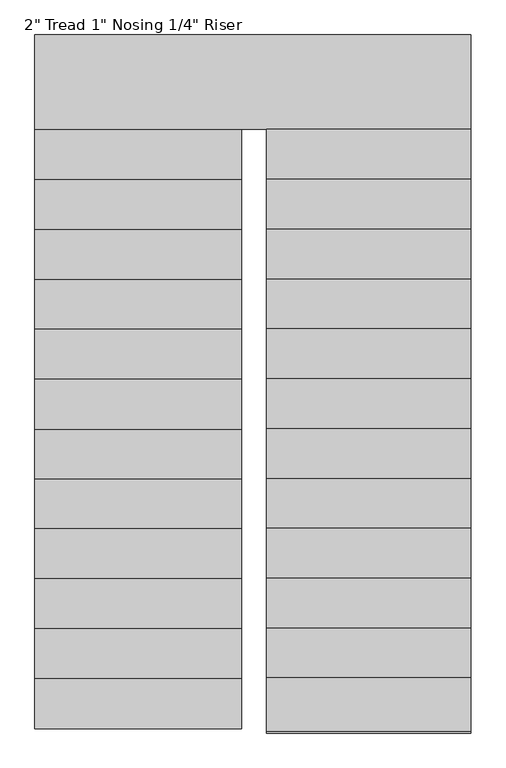
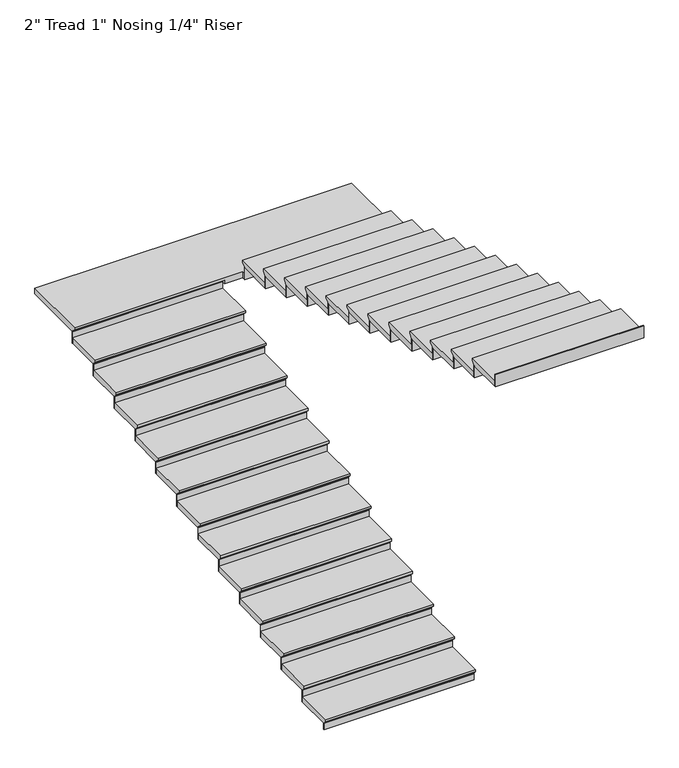
"""IFC4 building model written with IfcOpenShell, lengths in millimetres: stair flight geometry."""

from ifc_helpers import new_model, si_unit, origin, place, context, project, spatial, faceted_brep, source, transform, mapped, element, save


def stair_flight_f6874503(model_context):
    return source(origin(), model_context, "Body", "Brep", [
        faceted_brep([(-2593.7381751, -9955.5916506, 3134.4576923), (-2593.7381751, -9955.5916506, 3153.5076923), (-3857.687215, -9955.5916506, 3153.5076923), (-3857.687215, -9955.5916506, 3134.4576923), (-2593.7381751, -9930.1916506, 3109.0576923), (-3857.687215, -9930.1916506, 3109.0576923), (-2593.7381751, -9619.0416506, 3153.5076923), (-3857.687215, -9619.0416506, 3153.5076923), (-3857.687215, -9930.1916506, 3102.7076923), (-3857.687215, -9619.0416506, 3102.7076923), (-2593.7381751, -9619.0416506, 3102.7076923), (-2593.7381751, -9930.1916506, 3102.7076923)], [[[0, 1, 2, 3]], [[4, 0, 3, 5]], [[2, 1, 6, 7]], [[8, 9, 10, 11]], [[2, 7, 9, 8, 5, 3]], [[8, 11, 4, 5]], [[6, 1, 0, 4, 11, 10]], [[7, 6, 10, 9]]]),
        faceted_brep([(-2593.7381751, -9930.1916506, 3102.7076923), (-2593.7381751, -9930.1916506, 3048.0), (-2593.7381751, -9923.8416506, 3048.0), (-2593.7381751, -9923.8416506, 3102.7076923), (-3857.687215, -9930.1916506, 3102.7076923), (-3857.687215, -9923.8416506, 3102.7076923), (-3857.687215, -9923.8416506, 3048.0), (-3857.687215, -9930.1916506, 3048.0)], [[[0, 1, 2, 3]], [[4, 5, 6, 7]], [[1, 0, 4, 7]], [[2, 1, 7, 6]], [[3, 2, 6, 5]], [[0, 3, 5, 4]]]),
        faceted_brep([(-2593.7381751, -9619.0416506, 3208.2153846), (-2593.7381751, -9619.0416506, 3102.7076923), (-2593.7381751, -9612.6916506, 3102.7076923), (-2593.7381751, -9612.6916506, 3208.2153846), (-3857.687215, -9619.0416506, 3208.2153846), (-3857.687215, -9612.6916506, 3208.2153846), (-3857.687215, -9612.6916506, 3102.7076923), (-3857.687215, -9619.0416506, 3102.7076923)], [[[0, 1, 2, 3]], [[4, 5, 6, 7]], [[1, 0, 4, 7]], [[2, 1, 7, 6]], [[3, 2, 6, 5]], [[0, 3, 5, 4]]]),
        faceted_brep([(-3857.687215, -9644.4416506, 3259.0153846), (-2593.7381751, -9644.4416506, 3259.0153846), (-2593.7381751, -9314.2416506, 3259.0153846), (-3857.687215, -9314.2416506, 3259.0153846), (-3857.687215, -9619.0416506, 3208.2153846), (-3857.687215, -9314.2416506, 3208.2153846), (-2593.7381751, -9314.2416506, 3208.2153846), (-2593.7381751, -9619.0416506, 3208.2153846), (-3857.687215, -9619.0416506, 3214.5653846), (-3857.687215, -9644.4416506, 3239.9653846), (-2593.7381751, -9619.0416506, 3214.5653846), (-2593.7381751, -9644.4416506, 3239.9653846)], [[[0, 1, 2, 3]], [[4, 5, 6, 7]], [[0, 3, 5, 4, 8, 9]], [[4, 7, 10, 8]], [[2, 1, 11, 10, 7, 6]], [[3, 2, 6, 5]], [[11, 1, 0, 9]], [[10, 11, 9, 8]]]),
        faceted_brep([(-2593.7381751, -9314.2416506, 3313.7230769), (-2593.7381751, -9314.2416506, 3208.2153846), (-2593.7381751, -9307.8916506, 3208.2153846), (-2593.7381751, -9307.8916506, 3313.7230769), (-3857.687215, -9314.2416506, 3313.7230769), (-3857.687215, -9307.8916506, 3313.7230769), (-3857.687215, -9307.8916506, 3208.2153846), (-3857.687215, -9314.2416506, 3208.2153846)], [[[0, 1, 2, 3]], [[4, 5, 6, 7]], [[1, 0, 4, 7]], [[2, 1, 7, 6]], [[3, 2, 6, 5]], [[0, 3, 5, 4]]]),
        faceted_brep([(-3857.687215, -9339.6416506, 3364.5230769), (-2593.7381751, -9339.6416506, 3364.5230769), (-2593.7381751, -9009.4416506, 3364.5230769), (-3857.687215, -9009.4416506, 3364.5230769), (-3857.687215, -9314.2416506, 3313.7230769), (-3857.687215, -9009.4416506, 3313.7230769), (-2593.7381751, -9009.4416506, 3313.7230769), (-2593.7381751, -9314.2416506, 3313.7230769), (-3857.687215, -9314.2416506, 3320.0730769), (-3857.687215, -9339.6416506, 3345.4730769), (-2593.7381751, -9314.2416506, 3320.0730769), (-2593.7381751, -9339.6416506, 3345.4730769)], [[[0, 1, 2, 3]], [[4, 5, 6, 7]], [[0, 3, 5, 4, 8, 9]], [[4, 7, 10, 8]], [[2, 1, 11, 10, 7, 6]], [[3, 2, 6, 5]], [[11, 1, 0, 9]], [[10, 11, 9, 8]]]),
        faceted_brep([(-2593.7381751, -9009.4416506, 3419.2307692), (-2593.7381751, -9009.4416506, 3313.7230769), (-2593.7381751, -9003.0916506, 3313.7230769), (-2593.7381751, -9003.0916506, 3419.2307692), (-3857.687215, -9009.4416506, 3419.2307692), (-3857.687215, -9003.0916506, 3419.2307692), (-3857.687215, -9003.0916506, 3313.7230769), (-3857.687215, -9009.4416506, 3313.7230769)], [[[0, 1, 2, 3]], [[4, 5, 6, 7]], [[1, 0, 4, 7]], [[2, 1, 7, 6]], [[3, 2, 6, 5]], [[0, 3, 5, 4]]]),
        faceted_brep([(-3857.687215, -9034.8416506, 3470.0307692), (-2593.7381751, -9034.8416506, 3470.0307692), (-2593.7381751, -8704.6416506, 3470.0307692), (-3857.687215, -8704.6416506, 3470.0307692), (-3857.687215, -9009.4416506, 3419.2307692), (-3857.687215, -8704.6416506, 3419.2307692), (-2593.7381751, -8704.6416506, 3419.2307692), (-2593.7381751, -9009.4416506, 3419.2307692), (-3857.687215, -9009.4416506, 3425.5807692), (-3857.687215, -9034.8416506, 3450.9807692), (-2593.7381751, -9009.4416506, 3425.5807692), (-2593.7381751, -9034.8416506, 3450.9807692)], [[[0, 1, 2, 3]], [[4, 5, 6, 7]], [[0, 3, 5, 4, 8, 9]], [[4, 7, 10, 8]], [[2, 1, 11, 10, 7, 6]], [[3, 2, 6, 5]], [[11, 1, 0, 9]], [[10, 11, 9, 8]]]),
        faceted_brep([(-2593.7381751, -8704.6416506, 3524.7384615), (-2593.7381751, -8704.6416506, 3419.2307692), (-2593.7381751, -8698.2916506, 3419.2307692), (-2593.7381751, -8698.2916506, 3524.7384615), (-3857.687215, -8704.6416506, 3524.7384615), (-3857.687215, -8698.2916506, 3524.7384615), (-3857.687215, -8698.2916506, 3419.2307692), (-3857.687215, -8704.6416506, 3419.2307692)], [[[0, 1, 2, 3]], [[4, 5, 6, 7]], [[1, 0, 4, 7]], [[2, 1, 7, 6]], [[3, 2, 6, 5]], [[0, 3, 5, 4]]]),
        faceted_brep([(-3857.687215, -8730.0416506, 3575.5384615), (-2593.7381751, -8730.0416506, 3575.5384615), (-2593.7381751, -8399.8416506, 3575.5384615), (-3857.687215, -8399.8416506, 3575.5384615), (-3857.687215, -8704.6416506, 3524.7384615), (-3857.687215, -8399.8416506, 3524.7384615), (-2593.7381751, -8399.8416506, 3524.7384615), (-2593.7381751, -8704.6416506, 3524.7384615), (-3857.687215, -8704.6416506, 3531.0884615), (-3857.687215, -8730.0416506, 3556.4884615), (-2593.7381751, -8704.6416506, 3531.0884615), (-2593.7381751, -8730.0416506, 3556.4884615)], [[[0, 1, 2, 3]], [[4, 5, 6, 7]], [[0, 3, 5, 4, 8, 9]], [[4, 7, 10, 8]], [[2, 1, 11, 10, 7, 6]], [[3, 2, 6, 5]], [[11, 1, 0, 9]], [[10, 11, 9, 8]]]),
        faceted_brep([(-2593.7381751, -8399.8416506, 3630.2461538), (-2593.7381751, -8399.8416506, 3524.7384615), (-2593.7381751, -8393.4916506, 3524.7384615), (-2593.7381751, -8393.4916506, 3630.2461538), (-3857.687215, -8399.8416506, 3630.2461538), (-3857.687215, -8393.4916506, 3630.2461538), (-3857.687215, -8393.4916506, 3524.7384615), (-3857.687215, -8399.8416506, 3524.7384615)], [[[0, 1, 2, 3]], [[4, 5, 6, 7]], [[1, 0, 4, 7]], [[2, 1, 7, 6]], [[3, 2, 6, 5]], [[0, 3, 5, 4]]]),
        faceted_brep([(-3857.687215, -8425.2416506, 3681.0461538), (-2593.7381751, -8425.2416506, 3681.0461538), (-2593.7381751, -8098.2166506, 3681.0461538), (-3857.687215, -8098.2166506, 3681.0461538), (-3857.687215, -8399.8416506, 3630.2461538), (-3857.687215, -8098.2166506, 3630.2461538), (-2593.7381751, -8098.2166506, 3630.2461538), (-2593.7381751, -8399.8416506, 3630.2461538), (-3857.687215, -8399.8416506, 3636.5961538), (-3857.687215, -8425.2416506, 3661.9961538), (-2593.7381751, -8399.8416506, 3636.5961538), (-2593.7381751, -8425.2416506, 3661.9961538)], [[[0, 1, 2, 3]], [[4, 5, 6, 7]], [[0, 3, 5, 4, 8, 9]], [[4, 7, 10, 8]], [[2, 1, 11, 10, 7, 6]], [[3, 2, 6, 5]], [[11, 1, 0, 9]], [[10, 11, 9, 8]]]),
        faceted_brep([(-2593.7381751, -8098.2166506, 3735.7538462), (-2593.7381751, -8098.2166506, 3630.2461538), (-2593.7381751, -8091.8666506, 3630.2461538), (-2593.7381751, -8091.8666506, 3735.7538462), (-3857.687215, -8098.2166506, 3735.7538462), (-3857.687215, -8091.8666506, 3735.7538462), (-3857.687215, -8091.8666506, 3630.2461538), (-3857.687215, -8098.2166506, 3630.2461538)], [[[0, 1, 2, 3]], [[4, 5, 6, 7]], [[1, 0, 4, 7]], [[2, 1, 7, 6]], [[3, 2, 6, 5]], [[0, 3, 5, 4]]]),
        faceted_brep([(-3857.687215, -8123.6166506, 3786.5538462), (-2593.7381751, -8123.6166506, 3786.5538462), (-2593.7381751, -7790.2416506, 3786.5538462), (-3857.687215, -7790.2416506, 3786.5538462), (-3857.687215, -8098.2166506, 3735.7538462), (-3857.687215, -7790.2416506, 3735.7538462), (-2593.7381751, -7790.2416506, 3735.7538462), (-2593.7381751, -8098.2166506, 3735.7538462), (-3857.687215, -8098.2166506, 3742.1038462), (-3857.687215, -8123.6166506, 3767.5038462), (-2593.7381751, -8098.2166506, 3742.1038462), (-2593.7381751, -8123.6166506, 3767.5038462)], [[[0, 1, 2, 3]], [[4, 5, 6, 7]], [[0, 3, 5, 4, 8, 9]], [[4, 7, 10, 8]], [[2, 1, 11, 10, 7, 6]], [[3, 2, 6, 5]], [[11, 1, 0, 9]], [[10, 11, 9, 8]]]),
        faceted_brep([(-2593.7381751, -7790.2416506, 3841.2615385), (-2593.7381751, -7790.2416506, 3735.7538462), (-2593.7381751, -7783.8916506, 3735.7538462), (-2593.7381751, -7783.8916506, 3841.2615385), (-3857.687215, -7790.2416506, 3841.2615385), (-3857.687215, -7783.8916506, 3841.2615385), (-3857.687215, -7783.8916506, 3735.7538462), (-3857.687215, -7790.2416506, 3735.7538462)], [[[0, 1, 2, 3]], [[4, 5, 6, 7]], [[1, 0, 4, 7]], [[2, 1, 7, 6]], [[3, 2, 6, 5]], [[0, 3, 5, 4]]]),
        faceted_brep([(-3857.687215, -7815.6416506, 3892.0615385), (-2593.7381751, -7815.6416506, 3892.0615385), (-2593.7381751, -7485.4416506, 3892.0615385), (-3857.687215, -7485.4416506, 3892.0615385), (-3857.687215, -7790.2416506, 3841.2615385), (-3857.687215, -7485.4416506, 3841.2615385), (-2593.7381751, -7485.4416506, 3841.2615385), (-2593.7381751, -7790.2416506, 3841.2615385), (-3857.687215, -7790.2416506, 3847.6115385), (-3857.687215, -7815.6416506, 3873.0115385), (-2593.7381751, -7790.2416506, 3847.6115385), (-2593.7381751, -7815.6416506, 3873.0115385)], [[[0, 1, 2, 3]], [[4, 5, 6, 7]], [[0, 3, 5, 4, 8, 9]], [[4, 7, 10, 8]], [[2, 1, 11, 10, 7, 6]], [[3, 2, 6, 5]], [[11, 1, 0, 9]], [[10, 11, 9, 8]]]),
        faceted_brep([(-2593.7381751, -7485.4416506, 3946.7692308), (-2593.7381751, -7485.4416506, 3841.2615385), (-2593.7381751, -7479.0916506, 3841.2615385), (-2593.7381751, -7479.0916506, 3946.7692308), (-3857.687215, -7485.4416506, 3946.7692308), (-3857.687215, -7479.0916506, 3946.7692308), (-3857.687215, -7479.0916506, 3841.2615385), (-3857.687215, -7485.4416506, 3841.2615385)], [[[0, 1, 2, 3]], [[4, 5, 6, 7]], [[1, 0, 4, 7]], [[2, 1, 7, 6]], [[3, 2, 6, 5]], [[0, 3, 5, 4]]]),
        faceted_brep([(-3857.687215, -7510.8416506, 3997.5692308), (-2593.7381751, -7510.8416506, 3997.5692308), (-2593.7381751, -7180.6416506, 3997.5692308), (-3857.687215, -7180.6416506, 3997.5692308), (-3857.687215, -7485.4416506, 3946.7692308), (-3857.687215, -7180.6416506, 3946.7692308), (-2593.7381751, -7180.6416506, 3946.7692308), (-2593.7381751, -7485.4416506, 3946.7692308), (-3857.687215, -7485.4416506, 3953.1192308), (-3857.687215, -7510.8416506, 3978.5192308), (-2593.7381751, -7485.4416506, 3953.1192308), (-2593.7381751, -7510.8416506, 3978.5192308)], [[[0, 1, 2, 3]], [[4, 5, 6, 7]], [[0, 3, 5, 4, 8, 9]], [[4, 7, 10, 8]], [[2, 1, 11, 10, 7, 6]], [[3, 2, 6, 5]], [[11, 1, 0, 9]], [[10, 11, 9, 8]]]),
        faceted_brep([(-2593.7381751, -7180.6416506, 4052.2769231), (-2593.7381751, -7180.6416506, 3946.7692308), (-2593.7381751, -7174.2916506, 3946.7692308), (-2593.7381751, -7174.2916506, 4052.2769231), (-3857.687215, -7180.6416506, 4052.2769231), (-3857.687215, -7174.2916506, 4052.2769231), (-3857.687215, -7174.2916506, 3946.7692308), (-3857.687215, -7180.6416506, 3946.7692308)], [[[0, 1, 2, 3]], [[4, 5, 6, 7]], [[1, 0, 4, 7]], [[2, 1, 7, 6]], [[3, 2, 6, 5]], [[0, 3, 5, 4]]]),
        faceted_brep([(-3857.687215, -7206.0416506, 4103.0769231), (-2593.7381751, -7206.0416506, 4103.0769231), (-2593.7381751, -6875.8416506, 4103.0769231), (-3857.687215, -6875.8416506, 4103.0769231), (-3857.687215, -7180.6416506, 4052.2769231), (-3857.687215, -6875.8416506, 4052.2769231), (-2593.7381751, -6875.8416506, 4052.2769231), (-2593.7381751, -7180.6416506, 4052.2769231), (-3857.687215, -7180.6416506, 4058.6269231), (-3857.687215, -7206.0416506, 4084.0269231), (-2593.7381751, -7180.6416506, 4058.6269231), (-2593.7381751, -7206.0416506, 4084.0269231)], [[[0, 1, 2, 3]], [[4, 5, 6, 7]], [[0, 3, 5, 4, 8, 9]], [[4, 7, 10, 8]], [[2, 1, 11, 10, 7, 6]], [[3, 2, 6, 5]], [[11, 1, 0, 9]], [[10, 11, 9, 8]]]),
        faceted_brep([(-2593.7381751, -6875.8416506, 4157.7846154), (-2593.7381751, -6875.8416506, 4052.2769231), (-2593.7381751, -6869.4916506, 4052.2769231), (-2593.7381751, -6869.4916506, 4157.7846154), (-3857.687215, -6875.8416506, 4157.7846154), (-3857.687215, -6869.4916506, 4157.7846154), (-3857.687215, -6869.4916506, 4052.2769231), (-3857.687215, -6875.8416506, 4052.2769231)], [[[0, 1, 2, 3]], [[4, 5, 6, 7]], [[1, 0, 4, 7]], [[2, 1, 7, 6]], [[3, 2, 6, 5]], [[0, 3, 5, 4]]]),
        faceted_brep([(-3857.687215, -6901.2416506, 4208.5846154), (-2593.7381751, -6901.2416506, 4208.5846154), (-2593.7381751, -6571.0416506, 4208.5846154), (-3857.687215, -6571.0416506, 4208.5846154), (-3857.687215, -6875.8416506, 4157.7846154), (-3857.687215, -6571.0416506, 4157.7846154), (-2593.7381751, -6571.0416506, 4157.7846154), (-2593.7381751, -6875.8416506, 4157.7846154), (-3857.687215, -6875.8416506, 4164.1346154), (-3857.687215, -6901.2416506, 4189.5346154), (-2593.7381751, -6875.8416506, 4164.1346154), (-2593.7381751, -6901.2416506, 4189.5346154)], [[[0, 1, 2, 3]], [[4, 5, 6, 7]], [[0, 3, 5, 4, 8, 9]], [[4, 7, 10, 8]], [[2, 1, 11, 10, 7, 6]], [[3, 2, 6, 5]], [[11, 1, 0, 9]], [[10, 11, 9, 8]]]),
        faceted_brep([(-2593.7381751, -6571.0416506, 4263.2923077), (-2593.7381751, -6571.0416506, 4157.7846154), (-2593.7381751, -6564.6916506, 4157.7846154), (-2593.7381751, -6564.6916506, 4263.2923077), (-3857.687215, -6571.0416506, 4263.2923077), (-3857.687215, -6564.6916506, 4263.2923077), (-3857.687215, -6564.6916506, 4157.7846154), (-3857.687215, -6571.0416506, 4157.7846154)], [[[0, 1, 2, 3]], [[4, 5, 6, 7]], [[1, 0, 4, 7]], [[2, 1, 7, 6]], [[3, 2, 6, 5]], [[0, 3, 5, 4]]]),
        faceted_brep([(-3857.687215, -6596.4416506, 4314.0923077), (-2593.7381751, -6596.4416506, 4314.0923077), (-2593.7381751, -6266.2416506, 4314.0923077), (-3857.687215, -6266.2416506, 4314.0923077), (-3857.687215, -6571.0416506, 4263.2923077), (-3857.687215, -6266.2416506, 4263.2923077), (-2593.7381751, -6266.2416506, 4263.2923077), (-2593.7381751, -6571.0416506, 4263.2923077), (-3857.687215, -6571.0416506, 4269.6423077), (-3857.687215, -6596.4416506, 4295.0423077), (-2593.7381751, -6571.0416506, 4269.6423077), (-2593.7381751, -6596.4416506, 4295.0423077)], [[[0, 1, 2, 3]], [[4, 5, 6, 7]], [[0, 3, 5, 4, 8, 9]], [[4, 7, 10, 8]], [[2, 1, 11, 10, 7, 6]], [[3, 2, 6, 5]], [[11, 1, 0, 9]], [[10, 11, 9, 8]]]),
        faceted_brep([(-2593.7381751, -6266.2416506, 4368.8), (-2593.7381751, -6266.2416506, 4263.2923077), (-2593.7381751, -6259.8916506, 4263.2923077), (-2593.7381751, -6259.8916506, 4368.8), (-3857.687215, -6266.2416506, 4368.8), (-3857.687215, -6259.8916506, 4368.8), (-3857.687215, -6259.8916506, 4263.2923077), (-3857.687215, -6266.2416506, 4263.2923077)], [[[0, 1, 2, 3]], [[4, 5, 6, 7]], [[1, 0, 4, 7]], [[2, 1, 7, 6]], [[3, 2, 6, 5]], [[0, 3, 5, 4]]]),
        faceted_brep([(-1190.687215, -6317.0416506, 4419.6), (-1190.687215, -5713.7916506, 4419.6), (-3857.687215, -5713.7916506, 4419.6), (-3857.687215, -6291.6416506, 4419.6), (-2441.3381751, -6291.6416506, 4419.6), (-2441.3381751, -6317.0416506, 4419.6), (-1190.687215, -5713.7916506, 4368.8), (-1190.687215, -6317.0416506, 4368.8), (-2441.3381751, -6317.0416506, 4368.8), (-2441.3381751, -6291.6416506, 4368.8), (-2593.7381751, -6291.6416506, 4368.8), (-2593.7381751, -6266.2416506, 4368.8), (-3857.687215, -6266.2416506, 4368.8), (-3857.687215, -5713.7916506, 4368.8), (-3857.687215, -6266.2416506, 4375.15), (-3857.687215, -6291.6416506, 4400.55), (-2593.7381751, -6266.2416506, 4375.15), (-2593.7381751, -6291.6416506, 4400.55)], [[[0, 1, 2, 3, 4, 5]], [[6, 7, 8, 9, 10, 11, 12, 13]], [[1, 0, 7, 6]], [[2, 1, 6, 13]], [[3, 2, 13, 12, 14, 15]], [[12, 11, 16, 14]], [[11, 10, 17, 16]], [[4, 3, 15, 17, 10, 9]], [[5, 4, 9, 8]], [[0, 5, 8, 7]], [[15, 14, 16, 17]]]),
        faceted_brep([(-2441.3381751, -6317.0416506, 4474.3076923), (-2441.3381751, -6317.0416506, 4368.8), (-2441.3381751, -6323.3916506, 4368.8), (-2441.3381751, -6323.3916506, 4474.3076923), (-1190.687215, -6317.0416506, 4474.3076923), (-1190.687215, -6323.3916506, 4474.3076923), (-1190.687215, -6323.3916506, 4368.8), (-1190.687215, -6317.0416506, 4368.8)], [[[0, 1, 2, 3]], [[4, 5, 6, 7]], [[1, 0, 4, 7]], [[2, 1, 7, 6]], [[3, 2, 6, 5]], [[0, 3, 5, 4]]]),
        faceted_brep([(-1190.687215, -6291.6416506, 4525.1076923), (-2441.3381751, -6291.6416506, 4525.1076923), (-2441.3381751, -6621.8416506, 4525.1076923), (-1190.687215, -6621.8416506, 4525.1076923), (-1190.687215, -6317.0416506, 4474.3076923), (-1190.687215, -6621.8416506, 4474.3076923), (-2441.3381751, -6621.8416506, 4474.3076923), (-2441.3381751, -6317.0416506, 4474.3076923), (-1190.687215, -6317.0416506, 4480.6576923), (-1190.687215, -6291.6416506, 4506.0576923), (-2441.3381751, -6317.0416506, 4480.6576923), (-2441.3381751, -6291.6416506, 4506.0576923)], [[[0, 1, 2, 3]], [[4, 5, 6, 7]], [[0, 3, 5, 4, 8, 9]], [[4, 7, 10, 8]], [[2, 1, 11, 10, 7, 6]], [[3, 2, 6, 5]], [[11, 1, 0, 9]], [[10, 11, 9, 8]]]),
        faceted_brep([(-2441.3381751, -6621.8416506, 4579.8153846), (-2441.3381751, -6621.8416506, 4474.3076923), (-2441.3381751, -6628.1916506, 4474.3076923), (-2441.3381751, -6628.1916506, 4579.8153846), (-1190.687215, -6621.8416506, 4579.8153846), (-1190.687215, -6628.1916506, 4579.8153846), (-1190.687215, -6628.1916506, 4474.3076923), (-1190.687215, -6621.8416506, 4474.3076923)], [[[0, 1, 2, 3]], [[4, 5, 6, 7]], [[1, 0, 4, 7]], [[2, 1, 7, 6]], [[3, 2, 6, 5]], [[0, 3, 5, 4]]]),
        faceted_brep([(-1190.687215, -6596.4416506, 4630.6153846), (-2441.3381751, -6596.4416506, 4630.6153846), (-2441.3381751, -6926.6416506, 4630.6153846), (-1190.687215, -6926.6416506, 4630.6153846), (-1190.687215, -6621.8416506, 4579.8153846), (-1190.687215, -6926.6416506, 4579.8153846), (-2441.3381751, -6926.6416506, 4579.8153846), (-2441.3381751, -6621.8416506, 4579.8153846), (-1190.687215, -6621.8416506, 4586.1653846), (-1190.687215, -6596.4416506, 4611.5653846), (-2441.3381751, -6621.8416506, 4586.1653846), (-2441.3381751, -6596.4416506, 4611.5653846)], [[[0, 1, 2, 3]], [[4, 5, 6, 7]], [[0, 3, 5, 4, 8, 9]], [[4, 7, 10, 8]], [[2, 1, 11, 10, 7, 6]], [[3, 2, 6, 5]], [[11, 1, 0, 9]], [[10, 11, 9, 8]]]),
        faceted_brep([(-2441.3381751, -6926.6416506, 4685.3230769), (-2441.3381751, -6926.6416506, 4579.8153846), (-2441.3381751, -6932.9916506, 4579.8153846), (-2441.3381751, -6932.9916506, 4685.3230769), (-1190.687215, -6926.6416506, 4685.3230769), (-1190.687215, -6932.9916506, 4685.3230769), (-1190.687215, -6932.9916506, 4579.8153846), (-1190.687215, -6926.6416506, 4579.8153846)], [[[0, 1, 2, 3]], [[4, 5, 6, 7]], [[1, 0, 4, 7]], [[2, 1, 7, 6]], [[3, 2, 6, 5]], [[0, 3, 5, 4]]]),
        faceted_brep([(-1190.687215, -6901.2416506, 4736.1230769), (-2441.3381751, -6901.2416506, 4736.1230769), (-2441.3381751, -7231.4416506, 4736.1230769), (-1190.687215, -7231.4416506, 4736.1230769), (-1190.687215, -6926.6416506, 4685.3230769), (-1190.687215, -7231.4416506, 4685.3230769), (-2441.3381751, -7231.4416506, 4685.3230769), (-2441.3381751, -6926.6416506, 4685.3230769), (-1190.687215, -6926.6416506, 4691.6730769), (-1190.687215, -6901.2416506, 4717.0730769), (-2441.3381751, -6926.6416506, 4691.6730769), (-2441.3381751, -6901.2416506, 4717.0730769)], [[[0, 1, 2, 3]], [[4, 5, 6, 7]], [[0, 3, 5, 4, 8, 9]], [[4, 7, 10, 8]], [[2, 1, 11, 10, 7, 6]], [[3, 2, 6, 5]], [[11, 1, 0, 9]], [[10, 11, 9, 8]]]),
        faceted_brep([(-2441.3381751, -7231.4416506, 4790.8307692), (-2441.3381751, -7231.4416506, 4685.3230769), (-2441.3381751, -7237.7916506, 4685.3230769), (-2441.3381751, -7237.7916506, 4790.8307692), (-1190.687215, -7231.4416506, 4790.8307692), (-1190.687215, -7237.7916506, 4790.8307692), (-1190.687215, -7237.7916506, 4685.3230769), (-1190.687215, -7231.4416506, 4685.3230769)], [[[0, 1, 2, 3]], [[4, 5, 6, 7]], [[1, 0, 4, 7]], [[2, 1, 7, 6]], [[3, 2, 6, 5]], [[0, 3, 5, 4]]]),
        faceted_brep([(-1190.687215, -7206.0416506, 4841.6307692), (-2441.3381751, -7206.0416506, 4841.6307692), (-2441.3381751, -7536.2416506, 4841.6307692), (-1190.687215, -7536.2416506, 4841.6307692), (-1190.687215, -7231.4416506, 4790.8307692), (-1190.687215, -7536.2416506, 4790.8307692), (-2441.3381751, -7536.2416506, 4790.8307692), (-2441.3381751, -7231.4416506, 4790.8307692), (-1190.687215, -7231.4416506, 4797.1807692), (-1190.687215, -7206.0416506, 4822.5807692), (-2441.3381751, -7231.4416506, 4797.1807692), (-2441.3381751, -7206.0416506, 4822.5807692)], [[[0, 1, 2, 3]], [[4, 5, 6, 7]], [[0, 3, 5, 4, 8, 9]], [[4, 7, 10, 8]], [[2, 1, 11, 10, 7, 6]], [[3, 2, 6, 5]], [[11, 1, 0, 9]], [[10, 11, 9, 8]]]),
        faceted_brep([(-2441.3381751, -7536.2416506, 4896.3384615), (-2441.3381751, -7536.2416506, 4790.8307692), (-2441.3381751, -7542.5916506, 4790.8307692), (-2441.3381751, -7542.5916506, 4896.3384615), (-1190.687215, -7536.2416506, 4896.3384615), (-1190.687215, -7542.5916506, 4896.3384615), (-1190.687215, -7542.5916506, 4790.8307692), (-1190.687215, -7536.2416506, 4790.8307692)], [[[0, 1, 2, 3]], [[4, 5, 6, 7]], [[1, 0, 4, 7]], [[2, 1, 7, 6]], [[3, 2, 6, 5]], [[0, 3, 5, 4]]]),
        faceted_brep([(-1190.687215, -7510.8416506, 4947.1384615), (-2441.3381751, -7510.8416506, 4947.1384615), (-2441.3381751, -7841.0416506, 4947.1384615), (-1190.687215, -7841.0416506, 4947.1384615), (-1190.687215, -7536.2416506, 4896.3384615), (-1190.687215, -7841.0416506, 4896.3384615), (-2441.3381751, -7841.0416506, 4896.3384615), (-2441.3381751, -7536.2416506, 4896.3384615), (-1190.687215, -7536.2416506, 4902.6884615), (-1190.687215, -7510.8416506, 4928.0884615), (-2441.3381751, -7536.2416506, 4902.6884615), (-2441.3381751, -7510.8416506, 4928.0884615)], [[[0, 1, 2, 3]], [[4, 5, 6, 7]], [[0, 3, 5, 4, 8, 9]], [[4, 7, 10, 8]], [[2, 1, 11, 10, 7, 6]], [[3, 2, 6, 5]], [[11, 1, 0, 9]], [[10, 11, 9, 8]]]),
        faceted_brep([(-2441.3381751, -7841.0416506, 5001.8461538), (-2441.3381751, -7841.0416506, 4896.3384615), (-2441.3381751, -7847.3916506, 4896.3384615), (-2441.3381751, -7847.3916506, 5001.8461538), (-1190.687215, -7841.0416506, 5001.8461538), (-1190.687215, -7847.3916506, 5001.8461538), (-1190.687215, -7847.3916506, 4896.3384615), (-1190.687215, -7841.0416506, 4896.3384615)], [[[0, 1, 2, 3]], [[4, 5, 6, 7]], [[1, 0, 4, 7]], [[2, 1, 7, 6]], [[3, 2, 6, 5]], [[0, 3, 5, 4]]]),
        faceted_brep([(-1190.687215, -7815.6416506, 5052.6461538), (-2441.3381751, -7815.6416506, 5052.6461538), (-2441.3381751, -8145.8416506, 5052.6461538), (-1190.687215, -8145.8416506, 5052.6461538), (-1190.687215, -7841.0416506, 5001.8461538), (-1190.687215, -8145.8416506, 5001.8461538), (-2441.3381751, -8145.8416506, 5001.8461538), (-2441.3381751, -7841.0416506, 5001.8461538), (-1190.687215, -7841.0416506, 5008.1961538), (-1190.687215, -7815.6416506, 5033.5961538), (-2441.3381751, -7841.0416506, 5008.1961538), (-2441.3381751, -7815.6416506, 5033.5961538)], [[[0, 1, 2, 3]], [[4, 5, 6, 7]], [[0, 3, 5, 4, 8, 9]], [[4, 7, 10, 8]], [[2, 1, 11, 10, 7, 6]], [[3, 2, 6, 5]], [[11, 1, 0, 9]], [[10, 11, 9, 8]]]),
        faceted_brep([(-2441.3381751, -8145.8416506, 5107.3538462), (-2441.3381751, -8145.8416506, 5001.8461538), (-2441.3381751, -8152.1916506, 5001.8461538), (-2441.3381751, -8152.1916506, 5107.3538462), (-1190.687215, -8145.8416506, 5107.3538462), (-1190.687215, -8152.1916506, 5107.3538462), (-1190.687215, -8152.1916506, 5001.8461538), (-1190.687215, -8145.8416506, 5001.8461538)], [[[0, 1, 2, 3]], [[4, 5, 6, 7]], [[1, 0, 4, 7]], [[2, 1, 7, 6]], [[3, 2, 6, 5]], [[0, 3, 5, 4]]]),
        faceted_brep([(-1190.687215, -8120.4416506, 5158.1538462), (-2441.3381751, -8120.4416506, 5158.1538462), (-2441.3381751, -8450.6416506, 5158.1538462), (-1190.687215, -8450.6416506, 5158.1538462), (-1190.687215, -8145.8416506, 5107.3538462), (-1190.687215, -8450.6416506, 5107.3538462), (-2441.3381751, -8450.6416506, 5107.3538462), (-2441.3381751, -8145.8416506, 5107.3538462), (-1190.687215, -8145.8416506, 5113.7038462), (-1190.687215, -8120.4416506, 5139.1038462), (-2441.3381751, -8145.8416506, 5113.7038462), (-2441.3381751, -8120.4416506, 5139.1038462)], [[[0, 1, 2, 3]], [[4, 5, 6, 7]], [[0, 3, 5, 4, 8, 9]], [[4, 7, 10, 8]], [[2, 1, 11, 10, 7, 6]], [[3, 2, 6, 5]], [[11, 1, 0, 9]], [[10, 11, 9, 8]]]),
        faceted_brep([(-2441.3381751, -8450.6416506, 5212.8615385), (-2441.3381751, -8450.6416506, 5107.3538462), (-2441.3381751, -8456.9916506, 5107.3538462), (-2441.3381751, -8456.9916506, 5212.8615385), (-1190.687215, -8450.6416506, 5212.8615385), (-1190.687215, -8456.9916506, 5212.8615385), (-1190.687215, -8456.9916506, 5107.3538462), (-1190.687215, -8450.6416506, 5107.3538462)], [[[0, 1, 2, 3]], [[4, 5, 6, 7]], [[1, 0, 4, 7]], [[2, 1, 7, 6]], [[3, 2, 6, 5]], [[0, 3, 5, 4]]]),
        faceted_brep([(-1190.687215, -8425.2416506, 5263.6615385), (-2441.3381751, -8425.2416506, 5263.6615385), (-2441.3381751, -8755.4416506, 5263.6615385), (-1190.687215, -8755.4416506, 5263.6615385), (-1190.687215, -8450.6416506, 5212.8615385), (-1190.687215, -8755.4416506, 5212.8615385), (-2441.3381751, -8755.4416506, 5212.8615385), (-2441.3381751, -8450.6416506, 5212.8615385), (-1190.687215, -8450.6416506, 5219.2115385), (-1190.687215, -8425.2416506, 5244.6115385), (-2441.3381751, -8450.6416506, 5219.2115385), (-2441.3381751, -8425.2416506, 5244.6115385)], [[[0, 1, 2, 3]], [[4, 5, 6, 7]], [[0, 3, 5, 4, 8, 9]], [[4, 7, 10, 8]], [[2, 1, 11, 10, 7, 6]], [[3, 2, 6, 5]], [[11, 1, 0, 9]], [[10, 11, 9, 8]]]),
        faceted_brep([(-2441.3381751, -8755.4416506, 5318.3692308), (-2441.3381751, -8755.4416506, 5212.8615385), (-2441.3381751, -8761.7916506, 5212.8615385), (-2441.3381751, -8761.7916506, 5318.3692308), (-1190.687215, -8755.4416506, 5318.3692308), (-1190.687215, -8761.7916506, 5318.3692308), (-1190.687215, -8761.7916506, 5212.8615385), (-1190.687215, -8755.4416506, 5212.8615385)], [[[0, 1, 2, 3]], [[4, 5, 6, 7]], [[1, 0, 4, 7]], [[2, 1, 7, 6]], [[3, 2, 6, 5]], [[0, 3, 5, 4]]]),
        faceted_brep([(-1190.687215, -8730.0416506, 5369.1692308), (-2441.3381751, -8730.0416506, 5369.1692308), (-2441.3381751, -9060.2416506, 5369.1692308), (-1190.687215, -9060.2416506, 5369.1692308), (-1190.687215, -8755.4416506, 5318.3692308), (-1190.687215, -9060.2416506, 5318.3692308), (-2441.3381751, -9060.2416506, 5318.3692308), (-2441.3381751, -8755.4416506, 5318.3692308), (-1190.687215, -8755.4416506, 5324.7192308), (-1190.687215, -8730.0416506, 5350.1192308), (-2441.3381751, -8755.4416506, 5324.7192308), (-2441.3381751, -8730.0416506, 5350.1192308)], [[[0, 1, 2, 3]], [[4, 5, 6, 7]], [[0, 3, 5, 4, 8, 9]], [[4, 7, 10, 8]], [[2, 1, 11, 10, 7, 6]], [[3, 2, 6, 5]], [[11, 1, 0, 9]], [[10, 11, 9, 8]]]),
        faceted_brep([(-2441.3381751, -9060.2416506, 5423.8769231), (-2441.3381751, -9060.2416506, 5318.3692308), (-2441.3381751, -9066.5916506, 5318.3692308), (-2441.3381751, -9066.5916506, 5423.8769231), (-1190.687215, -9060.2416506, 5423.8769231), (-1190.687215, -9066.5916506, 5423.8769231), (-1190.687215, -9066.5916506, 5318.3692308), (-1190.687215, -9060.2416506, 5318.3692308)], [[[0, 1, 2, 3]], [[4, 5, 6, 7]], [[1, 0, 4, 7]], [[2, 1, 7, 6]], [[3, 2, 6, 5]], [[0, 3, 5, 4]]]),
        faceted_brep([(-1190.687215, -9034.8416506, 5474.6769231), (-2441.3381751, -9034.8416506, 5474.6769231), (-2441.3381751, -9365.0416506, 5474.6769231), (-1190.687215, -9365.0416506, 5474.6769231), (-1190.687215, -9060.2416506, 5423.8769231), (-1190.687215, -9365.0416506, 5423.8769231), (-2441.3381751, -9365.0416506, 5423.8769231), (-2441.3381751, -9060.2416506, 5423.8769231), (-1190.687215, -9060.2416506, 5430.2269231), (-1190.687215, -9034.8416506, 5455.6269231), (-2441.3381751, -9060.2416506, 5430.2269231), (-2441.3381751, -9034.8416506, 5455.6269231)], [[[0, 1, 2, 3]], [[4, 5, 6, 7]], [[0, 3, 5, 4, 8, 9]], [[4, 7, 10, 8]], [[2, 1, 11, 10, 7, 6]], [[3, 2, 6, 5]], [[11, 1, 0, 9]], [[10, 11, 9, 8]]]),
        faceted_brep([(-2441.3381751, -9365.0416506, 5529.3846154), (-2441.3381751, -9365.0416506, 5423.8769231), (-2441.3381751, -9371.3916506, 5423.8769231), (-2441.3381751, -9371.3916506, 5529.3846154), (-1190.687215, -9365.0416506, 5529.3846154), (-1190.687215, -9371.3916506, 5529.3846154), (-1190.687215, -9371.3916506, 5423.8769231), (-1190.687215, -9365.0416506, 5423.8769231)], [[[0, 1, 2, 3]], [[4, 5, 6, 7]], [[1, 0, 4, 7]], [[2, 1, 7, 6]], [[3, 2, 6, 5]], [[0, 3, 5, 4]]]),
        faceted_brep([(-1190.687215, -9339.6416506, 5580.1846154), (-2441.3381751, -9339.6416506, 5580.1846154), (-2441.3381751, -9669.8416506, 5580.1846154), (-1190.687215, -9669.8416506, 5580.1846154), (-1190.687215, -9365.0416506, 5529.3846154), (-1190.687215, -9669.8416506, 5529.3846154), (-2441.3381751, -9669.8416506, 5529.3846154), (-2441.3381751, -9365.0416506, 5529.3846154), (-1190.687215, -9365.0416506, 5535.7346154), (-1190.687215, -9339.6416506, 5561.1346154), (-2441.3381751, -9365.0416506, 5535.7346154), (-2441.3381751, -9339.6416506, 5561.1346154)], [[[0, 1, 2, 3]], [[4, 5, 6, 7]], [[0, 3, 5, 4, 8, 9]], [[4, 7, 10, 8]], [[2, 1, 11, 10, 7, 6]], [[3, 2, 6, 5]], [[11, 1, 0, 9]], [[10, 11, 9, 8]]]),
        faceted_brep([(-2441.3381751, -9669.8416506, 5634.8923077), (-2441.3381751, -9669.8416506, 5529.3846154), (-2441.3381751, -9676.1916506, 5529.3846154), (-2441.3381751, -9676.1916506, 5634.8923077), (-1190.687215, -9669.8416506, 5634.8923077), (-1190.687215, -9676.1916506, 5634.8923077), (-1190.687215, -9676.1916506, 5529.3846154), (-1190.687215, -9669.8416506, 5529.3846154)], [[[0, 1, 2, 3]], [[4, 5, 6, 7]], [[1, 0, 4, 7]], [[2, 1, 7, 6]], [[3, 2, 6, 5]], [[0, 3, 5, 4]]]),
        faceted_brep([(-2441.3381751, -9974.6416506, 5740.4), (-2441.3381751, -9974.6416506, 5634.8923077), (-2441.3381751, -9980.9916506, 5634.8923077), (-2441.3381751, -9980.9916506, 5740.4), (-1190.687215, -9974.6416506, 5740.4), (-1190.687215, -9980.9916506, 5740.4), (-1190.687215, -9980.9916506, 5634.8923077), (-1190.687215, -9974.6416506, 5634.8923077)], [[[0, 1, 2, 3]], [[4, 5, 6, 7]], [[1, 0, 4, 7]], [[2, 1, 7, 6]], [[3, 2, 6, 5]], [[0, 3, 5, 4]]]),
        faceted_brep([(-1190.687215, -9644.4416506, 5685.6923077), (-2441.3381751, -9644.4416506, 5685.6923077), (-2441.3381751, -9974.6416506, 5685.6923077), (-1190.687215, -9974.6416506, 5685.6923077), (-1190.687215, -9669.8416506, 5634.8923077), (-1190.687215, -9974.6416506, 5634.8923077), (-2441.3381751, -9974.6416506, 5634.8923077), (-2441.3381751, -9669.8416506, 5634.8923077), (-1190.687215, -9669.8416506, 5641.2423077), (-1190.687215, -9644.4416506, 5666.6423077), (-2441.3381751, -9669.8416506, 5641.2423077), (-2441.3381751, -9644.4416506, 5666.6423077)], [[[0, 1, 2, 3]], [[4, 5, 6, 7]], [[0, 3, 5, 4, 8, 9]], [[4, 7, 10, 8]], [[2, 1, 11, 10, 7, 6]], [[3, 2, 6, 5]], [[11, 1, 0, 9]], [[10, 11, 9, 8]]]),
    ])


if __name__ == "__main__":
    model = new_model("IFC4")
    model_context = context("Model", 3, world=origin())
    ifc_project = project(units=[si_unit("LENGTHUNIT", "METRE", prefix="MILLI")], contexts=[model_context])
    site = spatial("IfcSite", under=ifc_project)
    building = spatial("IfcBuilding", under=site)
    placement = place(None, origin())
    stair_flight_shape = stair_flight_f6874503(model_context)
    element("IfcStairFlight", 1, ObjectType="2\" Tread 1\" Nosing 1/4\" Riser", at=placement, inside=building, context=model_context, shape_type="MappedRepresentation", body=[
        mapped(stair_flight_shape, transform((0.0, 0.0, 0.0), x_axis=(1.0, 0.0, 0.0), y_axis=(0.0, 1.0, 0.0), z_axis=(0.0, 0.0, 1.0))),
    ])
    save(model, "model.ifc")
